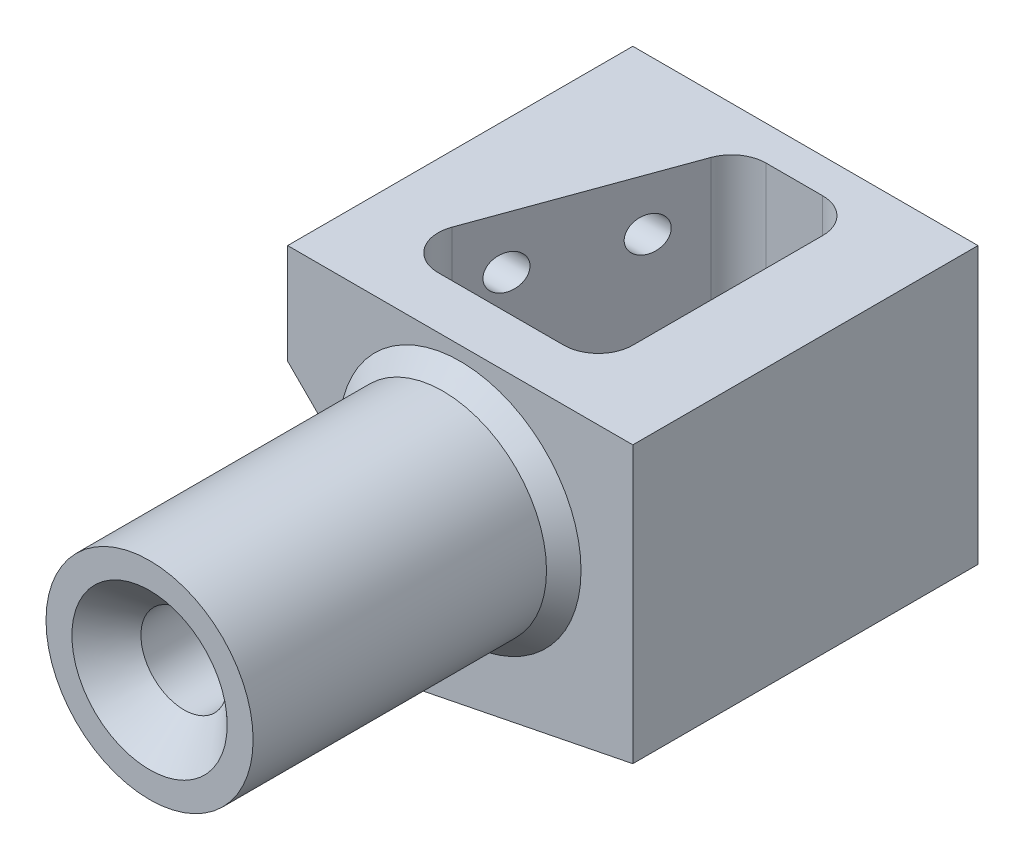
ISO-10303-21;
HEADER;
FILE_DESCRIPTION(('STEP AP214'),'2;1');
FILE_NAME('part.step','',(''),(''),'','','');
FILE_SCHEMA(('AUTOMOTIVE_DESIGN { 1 0 10303 214 1 1 1 1 }'));
ENDSEC;
DATA;
#1=APPLICATION_CONTEXT('core data for automotive mechanical design processes');
#2=APPLICATION_PROTOCOL_DEFINITION('international standard','automotive_design',2000,#1);
#3=PRODUCT_CONTEXT('',#1,'mechanical');
#4=PRODUCT('Part','Part','',(#3));
#5=PRODUCT_RELATED_PRODUCT_CATEGORY('part','',(#4));
#6=PRODUCT_DEFINITION_FORMATION('','',#4);
#7=PRODUCT_DEFINITION_CONTEXT('part definition',#1,'design');
#8=PRODUCT_DEFINITION('design','',#6,#7);
#9=PRODUCT_DEFINITION_SHAPE('','',#8);
#10=(LENGTH_UNIT() NAMED_UNIT(*) SI_UNIT(.MILLI.,.METRE.));
#11=(NAMED_UNIT(*) PLANE_ANGLE_UNIT() SI_UNIT($,.RADIAN.));
#12=(NAMED_UNIT(*) SI_UNIT($,.STERADIAN.) SOLID_ANGLE_UNIT());
#13=UNCERTAINTY_MEASURE_WITH_UNIT(LENGTH_MEASURE(1.E-05),#10,'distance_accuracy_value','');
#14=(GEOMETRIC_REPRESENTATION_CONTEXT(3) GLOBAL_UNCERTAINTY_ASSIGNED_CONTEXT((#13)) GLOBAL_UNIT_ASSIGNED_CONTEXT((#10,
#11,#12)) REPRESENTATION_CONTEXT('',''));
#15=CARTESIAN_POINT('',(0.,0.,0.));
#16=DIRECTION('',(0.,0.,1.));
#17=DIRECTION('',(1.,0.,0.));
#18=AXIS2_PLACEMENT_3D('',#15,#16,#17);
#19=CARTESIAN_POINT('',(0.,-10.,10.));
#20=DIRECTION('',(-0.196116135138184,0.98058067569092,0.));
#21=DIRECTION('',(-0.98058067569092,-0.196116135138184,0.));
#22=AXIS2_PLACEMENT_3D('',#19,#20,#21);
#23=PLANE('',#22);
#24=DIRECTION('',(0.98058067569092,0.196116135138184,0.));
#25=VECTOR('',#24,1.);
#26=CARTESIAN_POINT('',(0.,-10.,8.5));
#27=LINE('',#26,#25);
#28=CARTESIAN_POINT('',(2.85777798988684,-9.42844440202263,8.5));
#29=VERTEX_POINT('',#28);
#30=CARTESIAN_POINT('',(6.49999999999999,-8.7,8.5));
#31=VERTEX_POINT('',#30);
#32=EDGE_CURVE('E214',#29,#31,#27,.T.);
#33=ORIENTED_EDGE('',*,*,#32,.T.);
#34=CARTESIAN_POINT('',(6.5,-8.7,7.5));
#35=DIRECTION('',(-0.196116135138184,0.98058067569092,0.));
#36=DIRECTION('',(0.98058067569092,0.196116135138184,0.));
#37=AXIS2_PLACEMENT_3D('',#34,#35,#36);
#38=ELLIPSE('',#37,1.01980390271856,1.);
#39=CARTESIAN_POINT('',(7.5,-8.5,7.49999999999999));
#40=VERTEX_POINT('',#39);
#41=EDGE_CURVE('E217',#31,#40,#38,.T.);
#42=ORIENTED_EDGE('',*,*,#41,.T.);
#43=DIRECTION('',(0.,0.,-1.));
#44=VECTOR('',#43,1.);
#45=CARTESIAN_POINT('',(7.5,-8.5,10.));
#46=LINE('',#45,#44);
#47=CARTESIAN_POINT('',(7.5,-8.5,2.00000000000001));
#48=VERTEX_POINT('',#47);
#49=EDGE_CURVE('E187',#40,#48,#46,.T.);
#50=ORIENTED_EDGE('',*,*,#49,.T.);
#51=CARTESIAN_POINT('',(6.5,-8.7,2.));
#52=DIRECTION('',(-0.196116135138184,0.98058067569092,0.));
#53=DIRECTION('',(0.98058067569092,0.196116135138184,0.));
#54=AXIS2_PLACEMENT_3D('',#51,#52,#53);
#55=ELLIPSE('',#54,1.01980390271855,0.999999999999993);
#56=CARTESIAN_POINT('',(6.50000000000001,-8.7,1.00000000000001));
#57=VERTEX_POINT('',#56);
#58=EDGE_CURVE('E160',#48,#57,#55,.T.);
#59=ORIENTED_EDGE('',*,*,#58,.T.);
#60=DIRECTION('',(-0.98058067569092,-0.196116135138184,0.));
#61=VECTOR('',#60,1.);
#62=CARTESIAN_POINT('',(0.,-9.99999999999999,0.999999999999971));
#63=LINE('',#62,#61);
#64=CARTESIAN_POINT('',(4.85961427835095,-9.02807714432981,1.));
#65=VERTEX_POINT('',#64);
#66=EDGE_CURVE('E201',#57,#65,#63,.T.);
#67=ORIENTED_EDGE('',*,*,#66,.T.);
#68=CARTESIAN_POINT('',(4.85961427835094,-9.02807714432981,2.));
#69=DIRECTION('',(-0.196116135138184,0.98058067569092,0.));
#70=DIRECTION('',(0.98058067569092,0.196116135138184,0.));
#71=AXIS2_PLACEMENT_3D('',#68,#69,#70);
#72=ELLIPSE('',#71,1.01980390271855,0.999999999999998);
#73=CARTESIAN_POINT('',(3.91992165756503,-9.21601566848699,1.65797985667433));
#74=VERTEX_POINT('',#73);
#75=EDGE_CURVE('E206',#65,#74,#72,.T.);
#76=ORIENTED_EDGE('',*,*,#75,.T.);
#77=DIRECTION('',(-0.341222765371186,-0.0682445530742373,0.937501842861196));
#78=VECTOR('',#77,1.);
#79=CARTESIAN_POINT('',(0.776670210228654,-9.84466595795427,10.2939922318991));
#80=LINE('',#79,#78);
#81=CARTESIAN_POINT('',(1.91808536910092,-9.61638292617982,7.15797985667432));
#82=VERTEX_POINT('',#81);
#83=EDGE_CURVE('E207',#74,#82,#80,.T.);
#84=ORIENTED_EDGE('',*,*,#83,.T.);
#85=CARTESIAN_POINT('',(2.85777798988683,-9.42844440202263,7.5));
#86=DIRECTION('',(-0.196116135138184,0.98058067569092,0.));
#87=DIRECTION('',(0.98058067569092,0.196116135138184,0.));
#88=AXIS2_PLACEMENT_3D('',#85,#86,#87);
#89=ELLIPSE('',#88,1.01980390271856,1.);
#90=EDGE_CURVE('E215',#82,#29,#89,.T.);
#91=ORIENTED_EDGE('',*,*,#90,.T.);
#92=EDGE_LOOP('',(#33,#42,#50,#59,#67,#76,#84,#91));
#93=FACE_BOUND('',#92,.T.);
#94=DIRECTION('',(0.,0.,1.));
#95=VECTOR('',#94,1.);
#96=CARTESIAN_POINT('',(1.,-9.8,0.));
#97=LINE('',#96,#95);
#98=CARTESIAN_POINT('',(1.,-9.8,0.));
#99=VERTEX_POINT('',#98);
#100=CARTESIAN_POINT('',(1.,-9.8,10.));
#101=VERTEX_POINT('',#100);
#102=EDGE_CURVE('E234',#99,#101,#97,.T.);
#103=ORIENTED_EDGE('',*,*,#102,.F.);
#104=DIRECTION('',(0.98058067569092,0.196116135138184,0.));
#105=VECTOR('',#104,1.);
#106=CARTESIAN_POINT('',(0.,-10.,0.));
#107=LINE('',#106,#105);
#108=CARTESIAN_POINT('',(10.,-8.,0.));
#109=VERTEX_POINT('',#108);
#110=EDGE_CURVE('E254',#99,#109,#107,.T.);
#111=ORIENTED_EDGE('',*,*,#110,.T.);
#112=DIRECTION('',(0.,0.,-1.));
#113=VECTOR('',#112,1.);
#114=CARTESIAN_POINT('',(10.,-8.,10.));
#115=LINE('',#114,#113);
#116=CARTESIAN_POINT('',(10.,-8.,10.));
#117=VERTEX_POINT('',#116);
#118=EDGE_CURVE('E264',#117,#109,#115,.T.);
#119=ORIENTED_EDGE('',*,*,#118,.F.);
#120=DIRECTION('',(0.98058067569092,0.196116135138184,0.));
#121=VECTOR('',#120,1.);
#122=CARTESIAN_POINT('',(0.,-10.,10.));
#123=LINE('',#122,#121);
#124=EDGE_CURVE('E242',#101,#117,#123,.T.);
#125=ORIENTED_EDGE('',*,*,#124,.F.);
#126=EDGE_LOOP('',(#103,#111,#119,#125));
#127=FACE_BOUND('',#126,.T.);
#128=ADVANCED_FACE('F47',(#93,#127),#23,.F.);
#129=CARTESIAN_POINT('',(0.,0.,10.));
#130=DIRECTION('',(0.,0.,1.));
#131=DIRECTION('',(1.,0.,0.));
#132=AXIS2_PLACEMENT_3D('',#129,#130,#131);
#133=PLANE('',#132);
#134=CARTESIAN_POINT('',(5.,-3.90117401646231,10.));
#135=DIRECTION('',(0.,0.,1.));
#136=DIRECTION('',(1.,0.,0.));
#137=AXIS2_PLACEMENT_3D('',#134,#135,#136);
#138=CIRCLE('',#137,3.5);
#139=CARTESIAN_POINT('',(8.5,-3.90117401646231,10.));
#140=VERTEX_POINT('',#139);
#141=EDGE_CURVE('E279',#140,#140,#138,.F.);
#142=ORIENTED_EDGE('',*,*,#141,.T.);
#143=EDGE_LOOP('',(#142));
#144=FACE_BOUND('',#143,.T.);
#145=DIRECTION('',(-0.707106781186544,0.707106781186551,0.));
#146=VECTOR('',#145,1.);
#147=CARTESIAN_POINT('',(-1.45058700823115,-1.45058700823114,10.));
#148=LINE('',#147,#146);
#149=CARTESIAN_POINT('',(1.,-3.90117401646231,10.));
#150=VERTEX_POINT('',#149);
#151=CARTESIAN_POINT('',(0.,-2.9011740164623,10.));
#152=VERTEX_POINT('',#151);
#153=EDGE_CURVE('E223',#150,#152,#148,.T.);
#154=ORIENTED_EDGE('',*,*,#153,.F.);
#155=DIRECTION('',(0.,-1.,0.));
#156=VECTOR('',#155,1.);
#157=CARTESIAN_POINT('',(1.,0.,10.));
#158=LINE('',#157,#156);
#159=EDGE_CURVE('E222',#150,#101,#158,.T.);
#160=ORIENTED_EDGE('',*,*,#159,.T.);
#161=ORIENTED_EDGE('',*,*,#124,.T.);
#162=DIRECTION('',(0.,1.,0.));
#163=VECTOR('',#162,1.);
#164=CARTESIAN_POINT('',(10.,0.,10.));
#165=LINE('',#164,#163);
#166=CARTESIAN_POINT('',(10.,0.,10.));
#167=VERTEX_POINT('',#166);
#168=EDGE_CURVE('E247',#117,#167,#165,.T.);
#169=ORIENTED_EDGE('',*,*,#168,.T.);
#170=DIRECTION('',(-1.,0.,0.));
#171=VECTOR('',#170,1.);
#172=CARTESIAN_POINT('',(0.,0.,10.));
#173=LINE('',#172,#171);
#174=CARTESIAN_POINT('',(0.,0.,10.));
#175=VERTEX_POINT('',#174);
#176=EDGE_CURVE('E246',#167,#175,#173,.T.);
#177=ORIENTED_EDGE('',*,*,#176,.T.);
#178=DIRECTION('',(0.,-1.,0.));
#179=VECTOR('',#178,1.);
#180=CARTESIAN_POINT('',(0.,0.,10.));
#181=LINE('',#180,#179);
#182=EDGE_CURVE('E245',#175,#152,#181,.T.);
#183=ORIENTED_EDGE('',*,*,#182,.T.);
#184=EDGE_LOOP('',(#154,#160,#161,#169,#177,#183));
#185=FACE_BOUND('',#184,.T.);
#186=ADVANCED_FACE('F299',(#144,#185),#133,.T.);
#187=CARTESIAN_POINT('',(0.,0.,0.));
#188=DIRECTION('',(0.,0.,1.));
#189=DIRECTION('',(1.,0.,0.));
#190=AXIS2_PLACEMENT_3D('',#187,#188,#189);
#191=PLANE('',#190);
#192=DIRECTION('',(0.,-1.,0.));
#193=VECTOR('',#192,1.);
#194=CARTESIAN_POINT('',(1.,0.,0.));
#195=LINE('',#194,#193);
#196=CARTESIAN_POINT('',(1.,-3.90117401646231,0.));
#197=VERTEX_POINT('',#196);
#198=EDGE_CURVE('E225',#197,#99,#195,.T.);
#199=ORIENTED_EDGE('',*,*,#198,.F.);
#200=DIRECTION('',(-0.707106781186544,0.707106781186551,0.));
#201=VECTOR('',#200,1.);
#202=CARTESIAN_POINT('',(-1.45058700823115,-1.45058700823114,0.));
#203=LINE('',#202,#201);
#204=CARTESIAN_POINT('',(0.,-2.9011740164623,0.));
#205=VERTEX_POINT('',#204);
#206=EDGE_CURVE('E221',#197,#205,#203,.T.);
#207=ORIENTED_EDGE('',*,*,#206,.T.);
#208=DIRECTION('',(0.,-1.,0.));
#209=VECTOR('',#208,1.);
#210=CARTESIAN_POINT('',(0.,0.,0.));
#211=LINE('',#210,#209);
#212=CARTESIAN_POINT('',(0.,0.,0.));
#213=VERTEX_POINT('',#212);
#214=EDGE_CURVE('E243',#213,#205,#211,.T.);
#215=ORIENTED_EDGE('',*,*,#214,.F.);
#216=DIRECTION('',(-1.,0.,0.));
#217=VECTOR('',#216,1.);
#218=CARTESIAN_POINT('',(0.,0.,0.));
#219=LINE('',#218,#217);
#220=CARTESIAN_POINT('',(10.,0.,0.));
#221=VERTEX_POINT('',#220);
#222=EDGE_CURVE('E248',#221,#213,#219,.T.);
#223=ORIENTED_EDGE('',*,*,#222,.F.);
#224=DIRECTION('',(0.,1.,0.));
#225=VECTOR('',#224,1.);
#226=CARTESIAN_POINT('',(10.,0.,0.));
#227=LINE('',#226,#225);
#228=EDGE_CURVE('E260',#109,#221,#227,.T.);
#229=ORIENTED_EDGE('',*,*,#228,.F.);
#230=ORIENTED_EDGE('',*,*,#110,.F.);
#231=EDGE_LOOP('',(#199,#207,#215,#223,#229,#230));
#232=FACE_BOUND('',#231,.T.);
#233=ADVANCED_FACE('F307',(#232),#191,.F.);
#234=CARTESIAN_POINT('',(0.,0.,10.));
#235=DIRECTION('',(1.,0.,0.));
#236=DIRECTION('',(0.,0.,-1.));
#237=AXIS2_PLACEMENT_3D('',#234,#235,#236);
#238=PLANE('',#237);
#239=CARTESIAN_POINT('',(0.,-1.5,3.));
#240=DIRECTION('',(-1.,0.,0.));
#241=DIRECTION('',(0.,0.,1.));
#242=AXIS2_PLACEMENT_3D('',#239,#240,#241);
#243=CIRCLE('',#242,0.5);
#244=CARTESIAN_POINT('',(0.,-1.5,3.5));
#245=VERTEX_POINT('',#244);
#246=EDGE_CURVE('E272',#245,#245,#243,.T.);
#247=ORIENTED_EDGE('',*,*,#246,.F.);
#248=EDGE_LOOP('',(#247));
#249=FACE_BOUND('',#248,.T.);
#250=CARTESIAN_POINT('',(0.,-1.5,6.));
#251=DIRECTION('',(-1.,0.,0.));
#252=DIRECTION('',(0.,0.,1.));
#253=AXIS2_PLACEMENT_3D('',#250,#251,#252);
#254=CIRCLE('',#253,0.5);
#255=CARTESIAN_POINT('',(0.,-1.5,6.5));
#256=VERTEX_POINT('',#255);
#257=EDGE_CURVE('E281',#256,#256,#254,.T.);
#258=ORIENTED_EDGE('',*,*,#257,.F.);
#259=EDGE_LOOP('',(#258));
#260=FACE_BOUND('',#259,.T.);
#261=ORIENTED_EDGE('',*,*,#214,.T.);
#262=DIRECTION('',(0.,0.,1.));
#263=VECTOR('',#262,1.);
#264=CARTESIAN_POINT('',(0.,-2.9011740164623,0.));
#265=LINE('',#264,#263);
#266=EDGE_CURVE('E231',#205,#152,#265,.T.);
#267=ORIENTED_EDGE('',*,*,#266,.T.);
#268=ORIENTED_EDGE('',*,*,#182,.F.);
#269=DIRECTION('',(0.,0.,-1.));
#270=VECTOR('',#269,1.);
#271=CARTESIAN_POINT('',(0.,0.,10.));
#272=LINE('',#271,#270);
#273=EDGE_CURVE('E252',#175,#213,#272,.T.);
#274=ORIENTED_EDGE('',*,*,#273,.T.);
#275=EDGE_LOOP('',(#261,#267,#268,#274));
#276=FACE_BOUND('',#275,.T.);
#277=ADVANCED_FACE('F312',(#249,#260,#276),#238,.F.);
#278=CARTESIAN_POINT('',(10.,0.,10.));
#279=DIRECTION('',(-1.,0.,0.));
#280=DIRECTION('',(0.,0.,1.));
#281=AXIS2_PLACEMENT_3D('',#278,#279,#280);
#282=PLANE('',#281);
#283=ORIENTED_EDGE('',*,*,#228,.T.);
#284=DIRECTION('',(0.,0.,-1.));
#285=VECTOR('',#284,1.);
#286=CARTESIAN_POINT('',(10.,0.,10.));
#287=LINE('',#286,#285);
#288=EDGE_CURVE('E265',#167,#221,#287,.T.);
#289=ORIENTED_EDGE('',*,*,#288,.F.);
#290=ORIENTED_EDGE('',*,*,#168,.F.);
#291=ORIENTED_EDGE('',*,*,#118,.T.);
#292=EDGE_LOOP('',(#283,#289,#290,#291));
#293=FACE_BOUND('',#292,.T.);
#294=ADVANCED_FACE('F311',(#293),#282,.F.);
#295=CARTESIAN_POINT('',(0.,0.,10.));
#296=DIRECTION('',(0.,-1.,0.));
#297=DIRECTION('',(0.,0.,-1.));
#298=AXIS2_PLACEMENT_3D('',#295,#296,#297);
#299=PLANE('',#298);
#300=DIRECTION('',(0.,0.,-1.));
#301=VECTOR('',#300,1.);
#302=CARTESIAN_POINT('',(7.5,0.,7.49999999999999));
#303=LINE('',#302,#301);
#304=CARTESIAN_POINT('',(7.5,0.,7.49999999999999));
#305=VERTEX_POINT('',#304);
#306=CARTESIAN_POINT('',(7.49999999999999,0.,2.00000000000001));
#307=VERTEX_POINT('',#306);
#308=EDGE_CURVE('E162',#305,#307,#303,.T.);
#309=ORIENTED_EDGE('',*,*,#308,.F.);
#310=CARTESIAN_POINT('',(6.5,0.,7.5));
#311=DIRECTION('',(0.,1.,0.));
#312=DIRECTION('',(0.,0.,1.));
#313=AXIS2_PLACEMENT_3D('',#310,#311,#312);
#314=CIRCLE('',#313,1.);
#315=CARTESIAN_POINT('',(6.49999999999999,0.,8.5));
#316=VERTEX_POINT('',#315);
#317=EDGE_CURVE('E71',#316,#305,#314,.T.);
#318=ORIENTED_EDGE('',*,*,#317,.F.);
#319=DIRECTION('',(1.,0.,0.));
#320=VECTOR('',#319,1.);
#321=CARTESIAN_POINT('',(5.,0.,8.5));
#322=LINE('',#321,#320);
#323=CARTESIAN_POINT('',(2.85777798988684,0.,8.5));
#324=VERTEX_POINT('',#323);
#325=EDGE_CURVE('E183',#324,#316,#322,.T.);
#326=ORIENTED_EDGE('',*,*,#325,.F.);
#327=CARTESIAN_POINT('',(2.85777798988683,0.,7.5));
#328=DIRECTION('',(0.,1.,0.));
#329=DIRECTION('',(0.,0.,-1.));
#330=AXIS2_PLACEMENT_3D('',#327,#328,#329);
#331=CIRCLE('',#330,1.);
#332=CARTESIAN_POINT('',(1.91808536910092,0.,7.15797985667432));
#333=VERTEX_POINT('',#332);
#334=EDGE_CURVE('E185',#333,#324,#331,.T.);
#335=ORIENTED_EDGE('',*,*,#334,.F.);
#336=DIRECTION('',(-0.342020143325669,0.,0.939692620785908));
#337=VECTOR('',#336,1.);
#338=CARTESIAN_POINT('',(2.65076844803523,0.,5.14494964168583));
#339=LINE('',#338,#337);
#340=CARTESIAN_POINT('',(3.91992165756503,0.,1.65797985667433));
#341=VERTEX_POINT('',#340);
#342=EDGE_CURVE('E180',#341,#333,#339,.T.);
#343=ORIENTED_EDGE('',*,*,#342,.F.);
#344=CARTESIAN_POINT('',(4.85961427835094,0.,2.));
#345=DIRECTION('',(0.,1.,0.));
#346=DIRECTION('',(0.,0.,1.));
#347=AXIS2_PLACEMENT_3D('',#344,#345,#346);
#348=CIRCLE('',#347,0.999999999999998);
#349=CARTESIAN_POINT('',(4.85961427835095,0.,1.));
#350=VERTEX_POINT('',#349);
#351=EDGE_CURVE('E171',#350,#341,#348,.T.);
#352=ORIENTED_EDGE('',*,*,#351,.F.);
#353=DIRECTION('',(-1.,0.,0.));
#354=VECTOR('',#353,1.);
#355=CARTESIAN_POINT('',(6.50000000000001,0.,1.00000000000001));
#356=LINE('',#355,#354);
#357=CARTESIAN_POINT('',(6.50000000000001,0.,1.00000000000001));
#358=VERTEX_POINT('',#357);
#359=EDGE_CURVE('E173',#358,#350,#356,.T.);
#360=ORIENTED_EDGE('',*,*,#359,.F.);
#361=CARTESIAN_POINT('',(6.5,0.,2.));
#362=DIRECTION('',(0.,1.,0.));
#363=DIRECTION('',(0.,0.,1.));
#364=AXIS2_PLACEMENT_3D('',#361,#362,#363);
#365=CIRCLE('',#364,0.999999999999993);
#366=EDGE_CURVE('E152',#307,#358,#365,.T.);
#367=ORIENTED_EDGE('',*,*,#366,.F.);
#368=EDGE_LOOP('',(#309,#318,#326,#335,#343,#352,#360,#367));
#369=FACE_BOUND('',#368,.T.);
#370=ORIENTED_EDGE('',*,*,#222,.T.);
#371=ORIENTED_EDGE('',*,*,#273,.F.);
#372=ORIENTED_EDGE('',*,*,#176,.F.);
#373=ORIENTED_EDGE('',*,*,#288,.T.);
#374=EDGE_LOOP('',(#370,#371,#372,#373));
#375=FACE_BOUND('',#374,.T.);
#376=ADVANCED_FACE('F170',(#369,#375),#299,.F.);
#377=CARTESIAN_POINT('',(5.,-3.90117401646231,19.));
#378=DIRECTION('',(0.,0.,-1.));
#379=DIRECTION('',(-1.,0.,0.));
#380=AXIS2_PLACEMENT_3D('',#377,#378,#379);
#381=CYLINDRICAL_SURFACE('',#380,3.);
#382=CARTESIAN_POINT('',(5.,-3.90117401646231,10.5));
#383=DIRECTION('',(0.,0.,1.));
#384=DIRECTION('',(1.,0.,0.));
#385=AXIS2_PLACEMENT_3D('',#382,#383,#384);
#386=CIRCLE('',#385,3.);
#387=CARTESIAN_POINT('',(8.,-3.90117401646231,10.5));
#388=VERTEX_POINT('',#387);
#389=EDGE_CURVE('E268',#388,#388,#386,.T.);
#390=ORIENTED_EDGE('',*,*,#389,.T.);
#391=EDGE_LOOP('',(#390));
#392=FACE_BOUND('',#391,.T.);
#393=CARTESIAN_POINT('',(5.,-3.90117401646231,19.));
#394=DIRECTION('',(0.,0.,1.));
#395=DIRECTION('',(1.,0.,0.));
#396=AXIS2_PLACEMENT_3D('',#393,#394,#395);
#397=CIRCLE('',#396,3.);
#398=CARTESIAN_POINT('',(8.,-3.90117401646231,19.));
#399=VERTEX_POINT('',#398);
#400=EDGE_CURVE('E235',#399,#399,#397,.T.);
#401=ORIENTED_EDGE('',*,*,#400,.F.);
#402=EDGE_LOOP('',(#401));
#403=FACE_BOUND('',#402,.T.);
#404=ADVANCED_FACE('F331',(#392,#403),#381,.T.);
#405=CARTESIAN_POINT('',(0.,0.,19.));
#406=DIRECTION('',(0.,0.,1.));
#407=DIRECTION('',(1.,0.,0.));
#408=AXIS2_PLACEMENT_3D('',#405,#406,#407);
#409=PLANE('',#408);
#410=CARTESIAN_POINT('',(5.,-3.90117401646231,19.));
#411=DIRECTION('',(0.,0.,1.));
#412=DIRECTION('',(1.,0.,0.));
#413=AXIS2_PLACEMENT_3D('',#410,#411,#412);
#414=CIRCLE('',#413,2.25);
#415=CARTESIAN_POINT('',(7.25,-3.90117401646231,19.));
#416=VERTEX_POINT('',#415);
#417=EDGE_CURVE('E11',#416,#416,#414,.F.);
#418=ORIENTED_EDGE('',*,*,#417,.T.);
#419=EDGE_LOOP('',(#418));
#420=FACE_BOUND('',#419,.T.);
#421=ORIENTED_EDGE('',*,*,#400,.T.);
#422=EDGE_LOOP('',(#421));
#423=FACE_BOUND('',#422,.T.);
#424=ADVANCED_FACE('F340',(#420,#423),#409,.T.);
#425=CARTESIAN_POINT('',(1.,0.,0.));
#426=DIRECTION('',(-1.,0.,0.));
#427=DIRECTION('',(0.,-1.,0.));
#428=AXIS2_PLACEMENT_3D('',#425,#426,#427);
#429=PLANE('',#428);
#430=ORIENTED_EDGE('',*,*,#159,.F.);
#431=DIRECTION('',(0.,0.,1.));
#432=VECTOR('',#431,1.);
#433=CARTESIAN_POINT('',(1.,-3.90117401646231,0.));
#434=LINE('',#433,#432);
#435=EDGE_CURVE('E226',#197,#150,#434,.T.);
#436=ORIENTED_EDGE('',*,*,#435,.F.);
#437=ORIENTED_EDGE('',*,*,#198,.T.);
#438=ORIENTED_EDGE('',*,*,#102,.T.);
#439=EDGE_LOOP('',(#430,#436,#437,#438));
#440=FACE_BOUND('',#439,.T.);
#441=ADVANCED_FACE('F344',(#440),#429,.T.);
#442=CARTESIAN_POINT('',(-1.45058700823115,-1.45058700823114,0.));
#443=DIRECTION('',(0.707106781186551,0.707106781186544,0.));
#444=DIRECTION('',(-0.707106781186544,0.707106781186551,0.));
#445=AXIS2_PLACEMENT_3D('',#442,#443,#444);
#446=PLANE('',#445);
#447=ORIENTED_EDGE('',*,*,#153,.T.);
#448=ORIENTED_EDGE('',*,*,#266,.F.);
#449=ORIENTED_EDGE('',*,*,#206,.F.);
#450=ORIENTED_EDGE('',*,*,#435,.T.);
#451=EDGE_LOOP('',(#447,#448,#449,#450));
#452=FACE_BOUND('',#451,.T.);
#453=ADVANCED_FACE('F349',(#452),#446,.F.);
#454=CARTESIAN_POINT('',(6.5,-10.,7.5));
#455=DIRECTION('',(0.,1.,0.));
#456=DIRECTION('',(0.,0.,1.));
#457=AXIS2_PLACEMENT_3D('',#454,#455,#456);
#458=CYLINDRICAL_SURFACE('',#457,1.);
#459=DIRECTION('',(0.,1.,0.));
#460=VECTOR('',#459,1.);
#461=CARTESIAN_POINT('',(6.49999999999999,-10.,8.5));
#462=LINE('',#461,#460);
#463=EDGE_CURVE('E186',#31,#316,#462,.T.);
#464=ORIENTED_EDGE('',*,*,#463,.T.);
#465=ORIENTED_EDGE('',*,*,#317,.T.);
#466=DIRECTION('',(0.,1.,0.));
#467=VECTOR('',#466,1.);
#468=CARTESIAN_POINT('',(7.5,-10.,7.49999999999999));
#469=LINE('',#468,#467);
#470=EDGE_CURVE('E159',#40,#305,#469,.T.);
#471=ORIENTED_EDGE('',*,*,#470,.F.);
#472=ORIENTED_EDGE('',*,*,#41,.F.);
#473=EDGE_LOOP('',(#464,#465,#471,#472));
#474=FACE_BOUND('',#473,.T.);
#475=ADVANCED_FACE('F385',(#474),#458,.F.);
#476=CARTESIAN_POINT('',(5.,-10.,8.5));
#477=DIRECTION('',(0.,0.,1.));
#478=DIRECTION('',(1.,0.,0.));
#479=AXIS2_PLACEMENT_3D('',#476,#477,#478);
#480=PLANE('',#479);
#481=CARTESIAN_POINT('',(5.,-3.90117401646231,8.5));
#482=DIRECTION('',(0.,0.,1.));
#483=DIRECTION('',(1.,0.,0.));
#484=AXIS2_PLACEMENT_3D('',#481,#482,#483);
#485=CIRCLE('',#484,1.25);
#486=CARTESIAN_POINT('',(6.25,-3.90117401646231,8.5));
#487=VERTEX_POINT('',#486);
#488=EDGE_CURVE('E283',#487,#487,#485,.T.);
#489=ORIENTED_EDGE('',*,*,#488,.T.);
#490=EDGE_LOOP('',(#489));
#491=FACE_BOUND('',#490,.T.);
#492=DIRECTION('',(0.,1.,0.));
#493=VECTOR('',#492,1.);
#494=CARTESIAN_POINT('',(2.85777798988684,-10.,8.5));
#495=LINE('',#494,#493);
#496=EDGE_CURVE('E193',#29,#324,#495,.T.);
#497=ORIENTED_EDGE('',*,*,#496,.T.);
#498=ORIENTED_EDGE('',*,*,#325,.T.);
#499=ORIENTED_EDGE('',*,*,#463,.F.);
#500=ORIENTED_EDGE('',*,*,#32,.F.);
#501=EDGE_LOOP('',(#497,#498,#499,#500));
#502=FACE_BOUND('',#501,.T.);
#503=ADVANCED_FACE('F384',(#491,#502),#480,.F.);
#504=CARTESIAN_POINT('',(2.85777798988683,-10.,7.5));
#505=DIRECTION('',(0.,1.,0.));
#506=DIRECTION('',(0.,0.,1.));
#507=AXIS2_PLACEMENT_3D('',#504,#505,#506);
#508=CYLINDRICAL_SURFACE('',#507,1.);
#509=DIRECTION('',(0.,1.,0.));
#510=VECTOR('',#509,1.);
#511=CARTESIAN_POINT('',(1.91808536910092,-10.,7.15797985667432));
#512=LINE('',#511,#510);
#513=EDGE_CURVE('E192',#82,#333,#512,.T.);
#514=ORIENTED_EDGE('',*,*,#513,.T.);
#515=ORIENTED_EDGE('',*,*,#334,.T.);
#516=ORIENTED_EDGE('',*,*,#496,.F.);
#517=ORIENTED_EDGE('',*,*,#90,.F.);
#518=EDGE_LOOP('',(#514,#515,#516,#517));
#519=FACE_BOUND('',#518,.T.);
#520=ADVANCED_FACE('F401',(#519),#508,.F.);
#521=CARTESIAN_POINT('',(2.65076844803523,-10.,5.14494964168583));
#522=DIRECTION('',(-0.939692620785908,0.,-0.342020143325669));
#523=DIRECTION('',(-0.342020143325669,0.,0.939692620785908));
#524=AXIS2_PLACEMENT_3D('',#521,#522,#523);
#525=PLANE('',#524);
#526=CARTESIAN_POINT('',(3.43146627160883,-1.5,3.));
#527=DIRECTION('',(-0.939692620785908,0.,-0.342020143325669));
#528=DIRECTION('',(-0.342020143325669,0.,0.939692620785908));
#529=AXIS2_PLACEMENT_3D('',#526,#527,#528);
#530=ELLIPSE('',#529,0.532088886237956,0.5);
#531=CARTESIAN_POINT('',(3.24948115447573,-1.5,3.5));
#532=VERTEX_POINT('',#531);
#533=EDGE_CURVE('E275',#532,#532,#530,.T.);
#534=ORIENTED_EDGE('',*,*,#533,.T.);
#535=EDGE_LOOP('',(#534));
#536=FACE_BOUND('',#535,.T.);
#537=CARTESIAN_POINT('',(2.33955556881022,-1.5,6.));
#538=DIRECTION('',(-0.939692620785908,0.,-0.342020143325669));
#539=DIRECTION('',(-0.342020143325669,0.,0.939692620785908));
#540=AXIS2_PLACEMENT_3D('',#537,#538,#539);
#541=ELLIPSE('',#540,0.532088886237956,0.5);
#542=CARTESIAN_POINT('',(2.15757045167712,-1.5,6.5));
#543=VERTEX_POINT('',#542);
#544=EDGE_CURVE('E267',#543,#543,#541,.T.);
#545=ORIENTED_EDGE('',*,*,#544,.T.);
#546=EDGE_LOOP('',(#545));
#547=FACE_BOUND('',#546,.T.);
#548=DIRECTION('',(0.,1.,0.));
#549=VECTOR('',#548,1.);
#550=CARTESIAN_POINT('',(3.91992165756503,-10.,1.65797985667433));
#551=LINE('',#550,#549);
#552=EDGE_CURVE('E191',#74,#341,#551,.T.);
#553=ORIENTED_EDGE('',*,*,#552,.T.);
#554=ORIENTED_EDGE('',*,*,#342,.T.);
#555=ORIENTED_EDGE('',*,*,#513,.F.);
#556=ORIENTED_EDGE('',*,*,#83,.F.);
#557=EDGE_LOOP('',(#553,#554,#555,#556));
#558=FACE_BOUND('',#557,.T.);
#559=ADVANCED_FACE('F400',(#536,#547,#558),#525,.F.);
#560=CARTESIAN_POINT('',(4.85961427835094,-10.,2.));
#561=DIRECTION('',(0.,1.,0.));
#562=DIRECTION('',(0.,0.,1.));
#563=AXIS2_PLACEMENT_3D('',#560,#561,#562);
#564=CYLINDRICAL_SURFACE('',#563,0.999999999999998);
#565=DIRECTION('',(0.,1.,0.));
#566=VECTOR('',#565,1.);
#567=CARTESIAN_POINT('',(4.85961427835095,-10.,1.));
#568=LINE('',#567,#566);
#569=EDGE_CURVE('E197',#65,#350,#568,.T.);
#570=ORIENTED_EDGE('',*,*,#569,.T.);
#571=ORIENTED_EDGE('',*,*,#351,.T.);
#572=ORIENTED_EDGE('',*,*,#552,.F.);
#573=ORIENTED_EDGE('',*,*,#75,.F.);
#574=EDGE_LOOP('',(#570,#571,#572,#573));
#575=FACE_BOUND('',#574,.T.);
#576=ADVANCED_FACE('F392',(#575),#564,.F.);
#577=CARTESIAN_POINT('',(6.50000000000001,-10.,1.00000000000001));
#578=DIRECTION('',(0.,0.,-1.));
#579=DIRECTION('',(-1.,0.,0.));
#580=AXIS2_PLACEMENT_3D('',#577,#578,#579);
#581=PLANE('',#580);
#582=DIRECTION('',(0.,1.,0.));
#583=VECTOR('',#582,1.);
#584=CARTESIAN_POINT('',(6.50000000000001,-10.,1.00000000000001));
#585=LINE('',#584,#583);
#586=EDGE_CURVE('E157',#57,#358,#585,.T.);
#587=ORIENTED_EDGE('',*,*,#586,.T.);
#588=ORIENTED_EDGE('',*,*,#359,.T.);
#589=ORIENTED_EDGE('',*,*,#569,.F.);
#590=ORIENTED_EDGE('',*,*,#66,.F.);
#591=EDGE_LOOP('',(#587,#588,#589,#590));
#592=FACE_BOUND('',#591,.T.);
#593=ADVANCED_FACE('F395',(#592),#581,.F.);
#594=CARTESIAN_POINT('',(6.5,-10.,2.));
#595=DIRECTION('',(0.,1.,0.));
#596=DIRECTION('',(0.,0.,1.));
#597=AXIS2_PLACEMENT_3D('',#594,#595,#596);
#598=CYLINDRICAL_SURFACE('',#597,0.999999999999993);
#599=DIRECTION('',(0.,1.,0.));
#600=VECTOR('',#599,1.);
#601=CARTESIAN_POINT('',(7.49999999999999,-10.,2.00000000000001));
#602=LINE('',#601,#600);
#603=EDGE_CURVE('E62',#48,#307,#602,.T.);
#604=ORIENTED_EDGE('',*,*,#603,.T.);
#605=ORIENTED_EDGE('',*,*,#366,.T.);
#606=ORIENTED_EDGE('',*,*,#586,.F.);
#607=ORIENTED_EDGE('',*,*,#58,.F.);
#608=EDGE_LOOP('',(#604,#605,#606,#607));
#609=FACE_BOUND('',#608,.T.);
#610=ADVANCED_FACE('F151',(#609),#598,.F.);
#611=CARTESIAN_POINT('',(7.5,-10.,7.49999999999999));
#612=DIRECTION('',(1.,0.,0.));
#613=DIRECTION('',(0.,0.,-1.));
#614=AXIS2_PLACEMENT_3D('',#611,#612,#613);
#615=PLANE('',#614);
#616=ORIENTED_EDGE('',*,*,#470,.T.);
#617=ORIENTED_EDGE('',*,*,#308,.T.);
#618=ORIENTED_EDGE('',*,*,#603,.F.);
#619=ORIENTED_EDGE('',*,*,#49,.F.);
#620=EDGE_LOOP('',(#616,#617,#618,#619));
#621=FACE_BOUND('',#620,.T.);
#622=ADVANCED_FACE('F163',(#621),#615,.F.);
#623=CARTESIAN_POINT('',(5.,-1.5,6.));
#624=DIRECTION('',(-1.,0.,0.));
#625=DIRECTION('',(0.,0.,1.));
#626=AXIS2_PLACEMENT_3D('',#623,#624,#625);
#627=CYLINDRICAL_SURFACE('',#626,0.5);
#628=ORIENTED_EDGE('',*,*,#257,.T.);
#629=EDGE_LOOP('',(#628));
#630=FACE_BOUND('',#629,.T.);
#631=ORIENTED_EDGE('',*,*,#544,.F.);
#632=EDGE_LOOP('',(#631));
#633=FACE_BOUND('',#632,.T.);
#634=ADVANCED_FACE('F330',(#630,#633),#627,.F.);
#635=CARTESIAN_POINT('',(5.,-1.5,3.));
#636=DIRECTION('',(-1.,0.,0.));
#637=DIRECTION('',(0.,0.,1.));
#638=AXIS2_PLACEMENT_3D('',#635,#636,#637);
#639=CYLINDRICAL_SURFACE('',#638,0.5);
#640=ORIENTED_EDGE('',*,*,#246,.T.);
#641=EDGE_LOOP('',(#640));
#642=FACE_BOUND('',#641,.T.);
#643=ORIENTED_EDGE('',*,*,#533,.F.);
#644=EDGE_LOOP('',(#643));
#645=FACE_BOUND('',#644,.T.);
#646=ADVANCED_FACE('F325',(#642,#645),#639,.F.);
#647=CARTESIAN_POINT('',(5.,-3.90117401646231,10.5));
#648=DIRECTION('',(0.,0.,-1.));
#649=DIRECTION('',(-1.,0.,0.));
#650=AXIS2_PLACEMENT_3D('',#647,#648,#649);
#651=CONICAL_SURFACE('',#650,3.,0.785398163397445);
#652=ORIENTED_EDGE('',*,*,#141,.F.);
#653=EDGE_LOOP('',(#652));
#654=FACE_BOUND('',#653,.T.);
#655=ORIENTED_EDGE('',*,*,#389,.F.);
#656=EDGE_LOOP('',(#655));
#657=FACE_BOUND('',#656,.T.);
#658=ADVANCED_FACE('F293',(#654,#657),#651,.T.);
#659=CARTESIAN_POINT('',(5.,-3.90117401646231,7.));
#660=DIRECTION('',(0.,0.,1.));
#661=DIRECTION('',(1.,0.,0.));
#662=AXIS2_PLACEMENT_3D('',#659,#660,#661);
#663=CYLINDRICAL_SURFACE('',#662,1.25);
#664=CARTESIAN_POINT('',(5.,-3.90117401646231,18.));
#665=DIRECTION('',(0.,0.,1.));
#666=DIRECTION('',(1.,0.,0.));
#667=AXIS2_PLACEMENT_3D('',#664,#665,#666);
#668=CIRCLE('',#667,1.25);
#669=CARTESIAN_POINT('',(6.25,-3.90117401646231,18.));
#670=VERTEX_POINT('',#669);
#671=EDGE_CURVE('E59',#670,#670,#668,.T.);
#672=ORIENTED_EDGE('',*,*,#671,.T.);
#673=EDGE_LOOP('',(#672));
#674=FACE_BOUND('',#673,.T.);
#675=ORIENTED_EDGE('',*,*,#488,.F.);
#676=EDGE_LOOP('',(#675));
#677=FACE_BOUND('',#676,.T.);
#678=ADVANCED_FACE('F289',(#674,#677),#663,.F.);
#679=CARTESIAN_POINT('',(5.,-3.90117401646231,18.));
#680=DIRECTION('',(0.,0.,1.));
#681=DIRECTION('',(1.,0.,0.));
#682=AXIS2_PLACEMENT_3D('',#679,#680,#681);
#683=CONICAL_SURFACE('',#682,1.25,0.78539816339745);
#684=ORIENTED_EDGE('',*,*,#417,.F.);
#685=EDGE_LOOP('',(#684));
#686=FACE_BOUND('',#685,.T.);
#687=ORIENTED_EDGE('',*,*,#671,.F.);
#688=EDGE_LOOP('',(#687));
#689=FACE_BOUND('',#688,.T.);
#690=ADVANCED_FACE('F55',(#686,#689),#683,.F.);
#691=CLOSED_SHELL('',(#128,#186,#233,#277,#294,#376,#404,#424,#441,#453,#475,#503,#520,#559,
#576,#593,#610,#622,#634,#646,#658,#678,#690));
#692=MANIFOLD_SOLID_BREP('B2',#691);
#693=ADVANCED_BREP_SHAPE_REPRESENTATION('',(#18,#692),#14);
#694=SHAPE_DEFINITION_REPRESENTATION(#9,#693);
ENDSEC;
END-ISO-10303-21;
